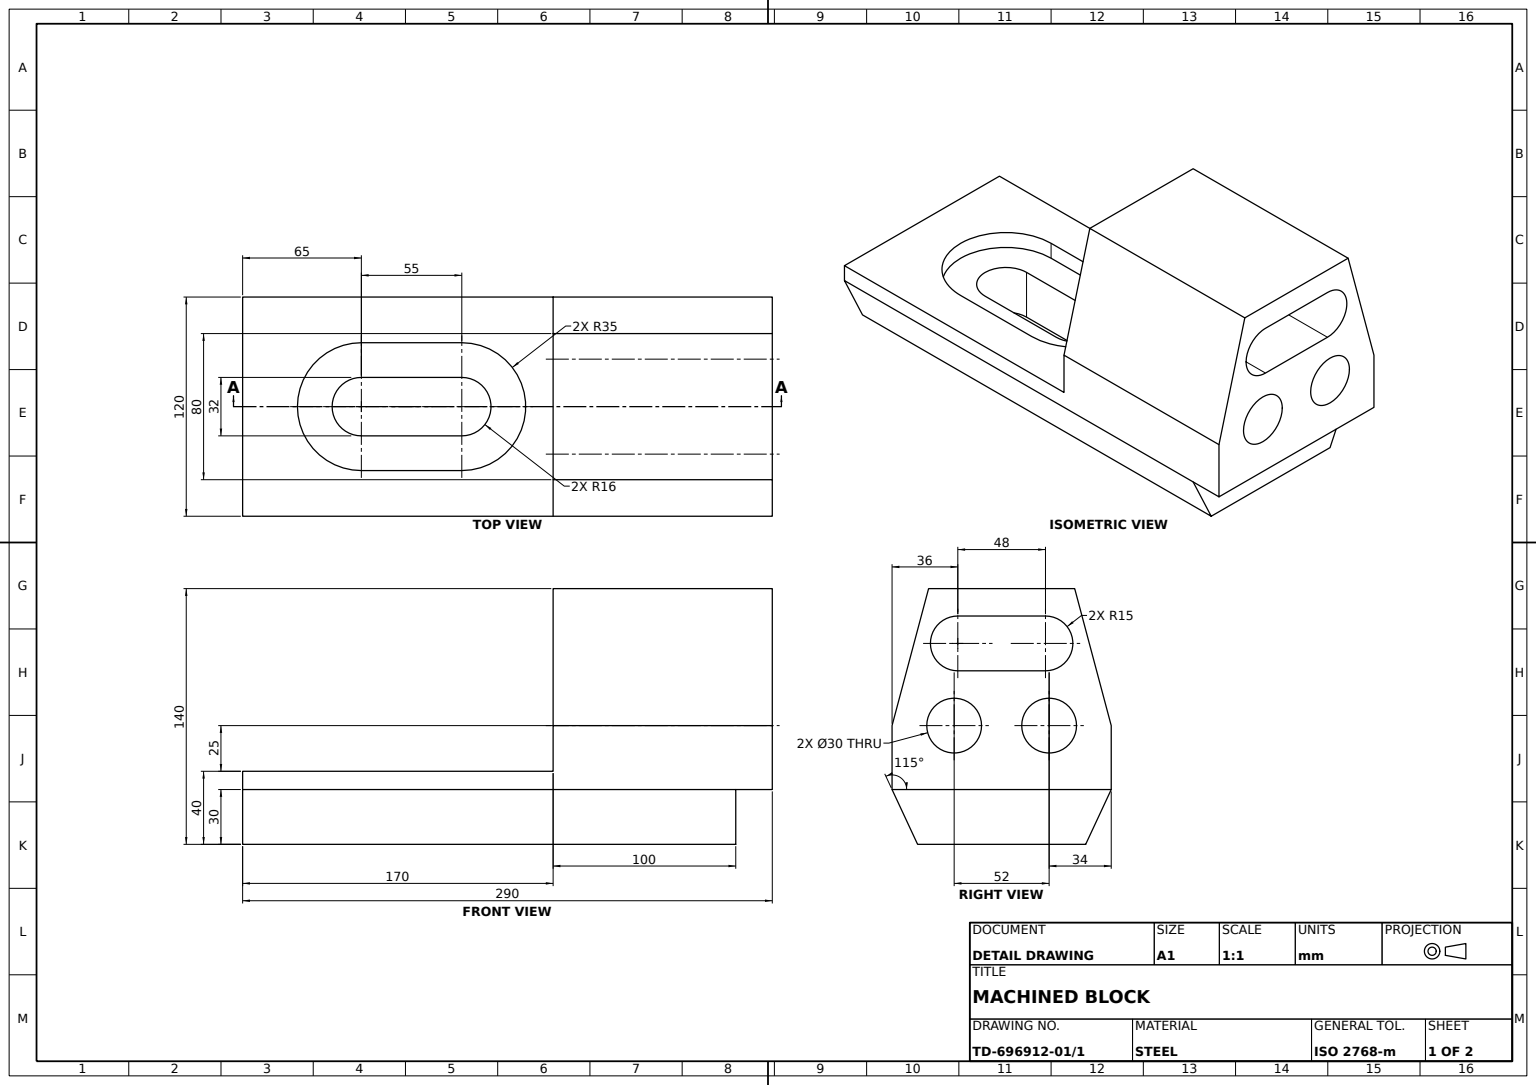
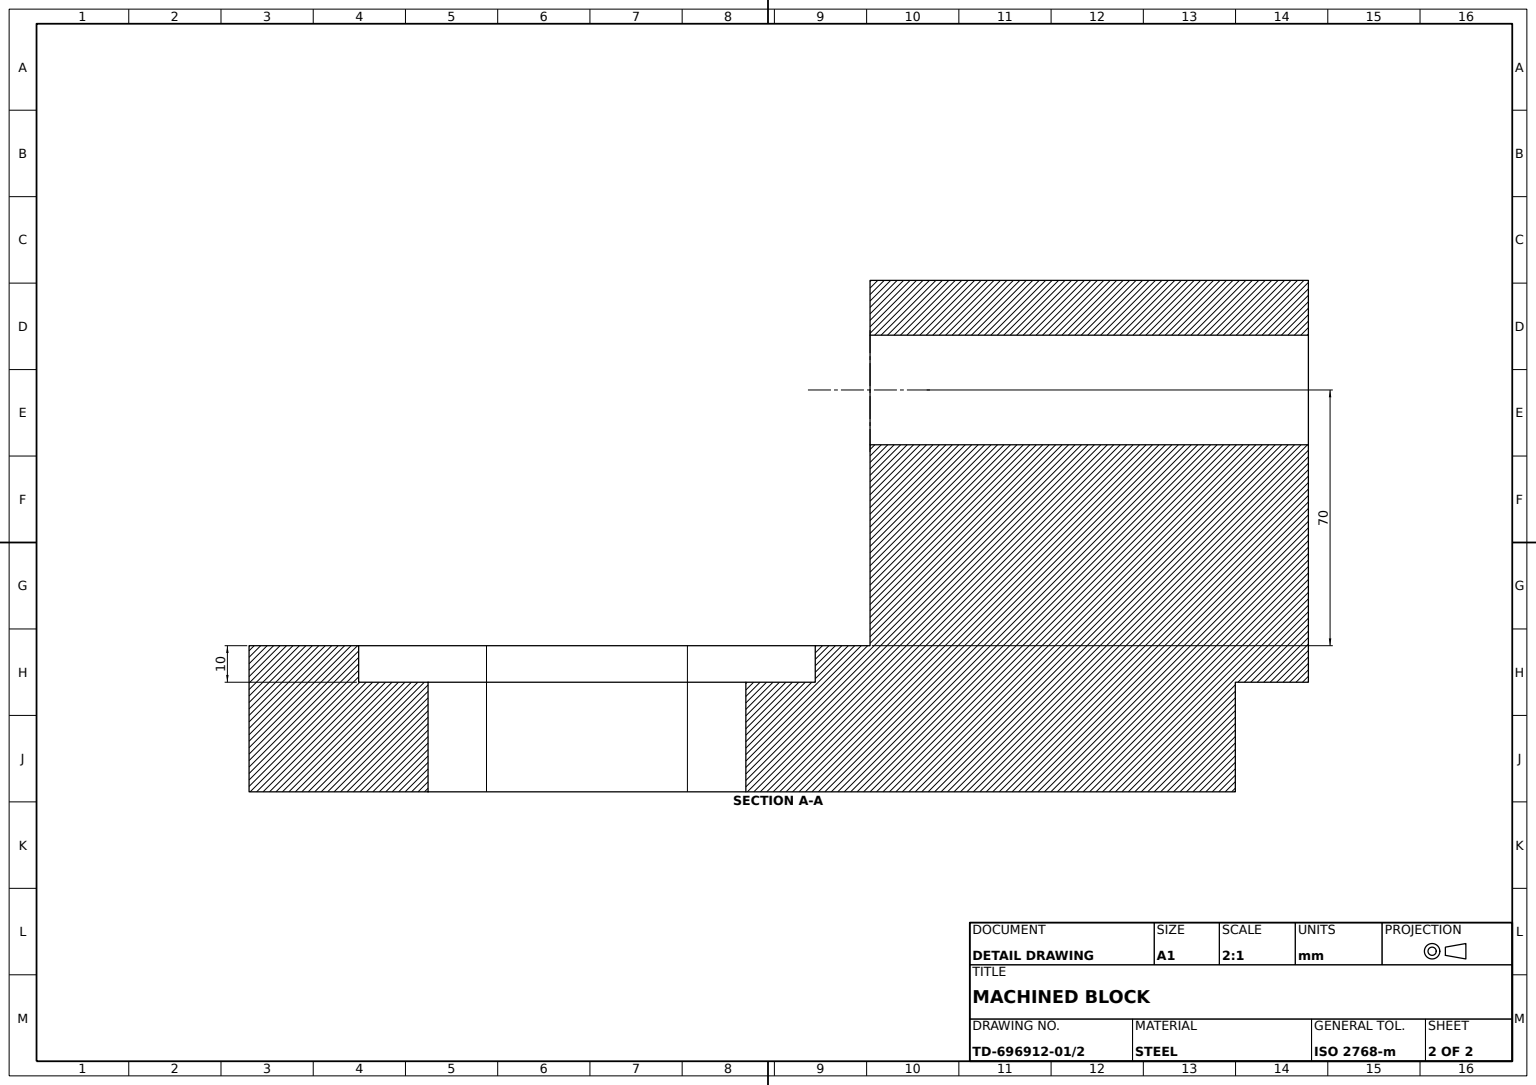
from build123d import *

# Parameters (mm, degrees)
BASE_RAIL_DEPTH                         = 170
BASE_RAIL_DEPTH_BACK                    = 100
UPRIGHT_BLOCK_PROFILE_SKETCH_R          = 15
UPRIGHT_BLOCK_WITH_SLOT_AND_HOLES_DEPTH = 120
UPRIGHT_EXTENSION_SKETCH_W              = 120
UPRIGHT_EXTENSION_SKETCH_H              = 10
UPRIGHT_EXTENSION_BLOCK_DEPTH           = 20
MOUNTING_SLOT_COUNTERBORE_10MM_DEPTH    = 10
MOUNTING_SLOT_THROUGH_REACH             = 208.155


with BuildPart() as part:
    # Base Rail Profile Sketch → Base Rail (new, two sides: drawn at the far end of the back side and taken through both)
    with BuildSketch(Plane.XY.offset(-BASE_RAIL_DEPTH_BACK)):
        Polygon((-46.010770255, 0), (46.010770255, 0), (60, 30), (60, 40), (-60, 40), (-60, 30), align=None)
    extrude(amount=BASE_RAIL_DEPTH + BASE_RAIL_DEPTH_BACK)

    # Upright Block Profile Sketch → Upright Block with Slot and Holes (add)
    with BuildSketch(Plane.XY):
        Polygon((-60, 40), (-60, 65), (-40, 140), (40, 140), (60, 65), (60, 40), align=None)
        with Locations((-26, 65)):
            Circle(UPRIGHT_BLOCK_PROFILE_SKETCH_R, mode=Mode.SUBTRACT)
        with Locations((26, 65)):
            Circle(UPRIGHT_BLOCK_PROFILE_SKETCH_R, mode=Mode.SUBTRACT)
        with BuildLine():
            Line((-24, 125), (24, 125))
            ThreePointArc((24, 125), (39, 110), (24, 95))
            Line((24, 95), (-24, 95))
            ThreePointArc((-24, 95), (-39, 110), (-24, 125))
        make_face(mode=Mode.SUBTRACT)
    extrude(amount=-UPRIGHT_BLOCK_WITH_SLOT_AND_HOLES_DEPTH)

    # Upright Extension Sketch → Upright Extension Block (add)
    with BuildSketch(Plane(origin=(0, 0, -100), x_dir=(-1, 0, 0), z_dir=(0, 0, -1))):
        with Locations((0, 35)):
            Rectangle(UPRIGHT_EXTENSION_SKETCH_W, UPRIGHT_EXTENSION_SKETCH_H)
    extrude(amount=UPRIGHT_EXTENSION_BLOCK_DEPTH)

    # Base Mounting Slot Sketch → Mounting Slot Counterbore 10mm (cut)
    with BuildSketch(Plane(origin=(0, 40, 0), x_dir=(1, 0, 0), z_dir=(0, 1, 0))):
        with BuildLine():
            Line((35, -50), (35, -105))
            ThreePointArc((35, -105), (0, -140), (-35, -105))
            Line((-35, -105), (-35, -50))
            ThreePointArc((-35, -50), (0, -15), (35, -50))
        make_face()
    extrude(amount=-MOUNTING_SLOT_COUNTERBORE_10MM_DEPTH, mode=Mode.SUBTRACT)

    # Sketch4_3 → Mounting Slot Through (cut, up to next)
    with BuildSketch(Plane(origin=(0, 40, 0), x_dir=(1, 0, 0), z_dir=(0, 1, 0)), mode=Mode.PRIVATE) as mounting_slot_through_sk1:
        with BuildLine():
            Line((16, -50), (16, -105))
            ThreePointArc((16, -105), (0, -121), (-16, -105))
            Line((-16, -105), (-16, -50))
            ThreePointArc((-16, -50), (0, -34), (16, -50))
        make_face()
    mounting_slot_through_tool1 = extrude(mounting_slot_through_sk1.sketch, amount=-MOUNTING_SLOT_THROUGH_REACH, mode=Mode.PRIVATE) & part.part
    add(mounting_slot_through_tool1.solids().sort_by_distance((0, 40, 77.5))[0], mode=Mode.SUBTRACT)


solid = part.part
